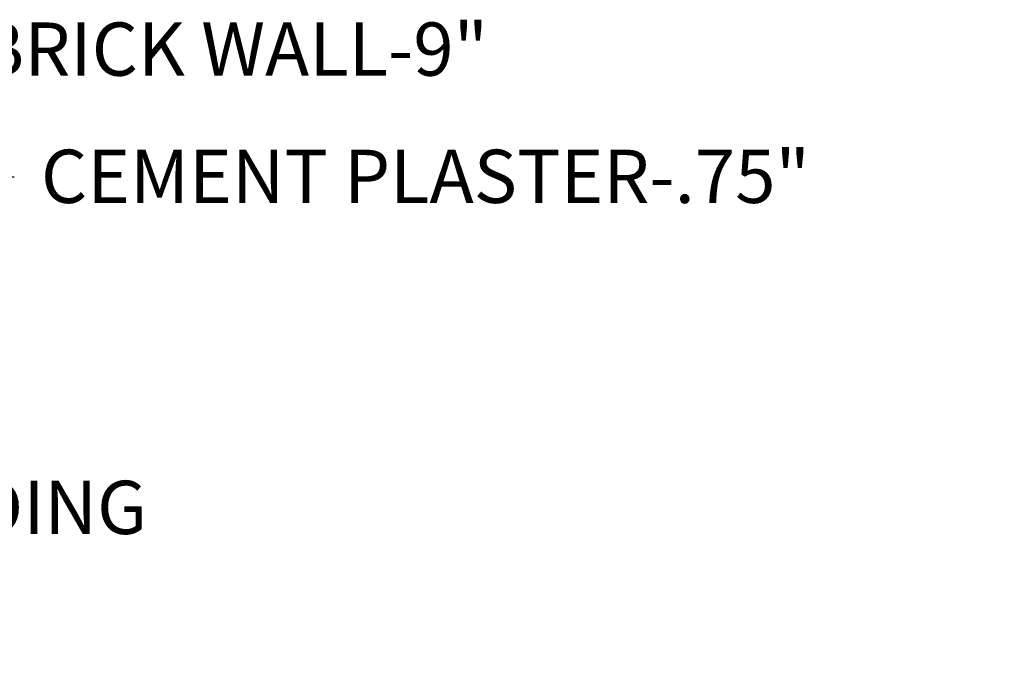
# Model space of a CAD drawing. Units: inches. Extents: x 2205 to 2524, y 4609 to 4803.
# Tile 5 of 5: x 2450 to 2524, y 4714 to 4762. Entities that reach past the tile are written whole.
import ezdxf
from ezdxf import colors
from ezdxf.entities.mleader import LeaderData, LeaderLine
from ezdxf.math import Vec2, Vec3

# ---------------------------------------------------------------- set-up
doc = ezdxf.new("R2010")
doc.units = ezdxf.units.IN
doc.layers.add('A-ANNO-SYMB', color=3, linetype='Continuous', lineweight=18)
doc.styles.get("Standard").update_dxf_attribs({"font": 'arial.ttf'})

msp = doc.modelspace()

# ---------------------------------------------------------------- leaders
at = {"layer": 'A-ANNO-SYMB'}
ml = msp.add_multileader_mtext('Standard', dxfattribs=at)
ml.set_content('BRICK WALL-9"', color=256)
ml.set_leader_properties()
ml.build(insert=Vec2(0, 0))
ctx = ml.context
ctx.base_point, ctx.plane_origin = Vec3(2444.382, 4760.141), Vec3(2424.362, 4760.141)
notes = []
notes.append((ctx, [(0, (1, 1, 0), (2436.382, 4760.141), (1, 0), 8, [(0, [(2424.362, 4760.141)], 0, [])])]))
ctx.mtext.insert, ctx.mtext.width, ctx.mtext.flow_direction = Vec3(2446.382, 4762.175), 53.5271, 5
ml = msp.add_multileader_mtext('Standard', dxfattribs=at)
ml.set_content('CEMENT PLASTER-.75"', color=256)
ml.set_leader_properties()
ml.build(insert=Vec2(0, 0))
ctx = ml.context
ctx.base_point, ctx.plane_origin = Vec3(2449.217, 4750.587), Vec3(2429.197, 4750.587)
notes.append((ctx, [(0, (1, 1, 0), (2441.217, 4750.587), (1, 0), 8, [(0, [(2429.197, 4750.587)], 0, [])])]))
ctx.mtext.insert, ctx.mtext.width, ctx.mtext.flow_direction = Vec3(2451.217, 4752.621), 72.36954, 5
ml = msp.add_multileader_mtext('Standard', dxfattribs=at)
ml.set_content('LANDING', color=256)
ml.set_leader_properties()
ml.build(insert=Vec2(0, 0))
ctx = ml.context
ctx.base_point, ctx.plane_origin = Vec3(2433.905, 4725.727), Vec3(2415.06, 4713.979)
notes.append((ctx, [(0, (1, 1, 0), (2415.06, 4725.727), (1, 0), 18.845, [(0, [(2415.06, 4713.979)], 0, [])])]))
ctx.mtext.insert, ctx.mtext.width, ctx.mtext.flow_direction = Vec3(2435.905, 4727.761), 24.36409, 5
for ctx, leaders in notes:
    for number, flags, end, landing, length, lines in leaders:
        leader = LeaderData()
        leader.index, (leader.has_last_leader_line, leader.has_dogleg_vector, leader.attachment_direction) = number, flags
        leader.last_leader_point, leader.dogleg_vector, leader.dogleg_length = Vec3(end), Vec3(landing), length
        for number, points, colour, breaks in lines:
            line = LeaderLine()
            line.index, line.vertices, line.color, line.breaks = number, Vec3.list(points), colors.encode_raw_color(colour), breaks
            leader.lines.append(line)
        ctx.leaders.append(leader)

doc.saveas('drawing.dxf')
